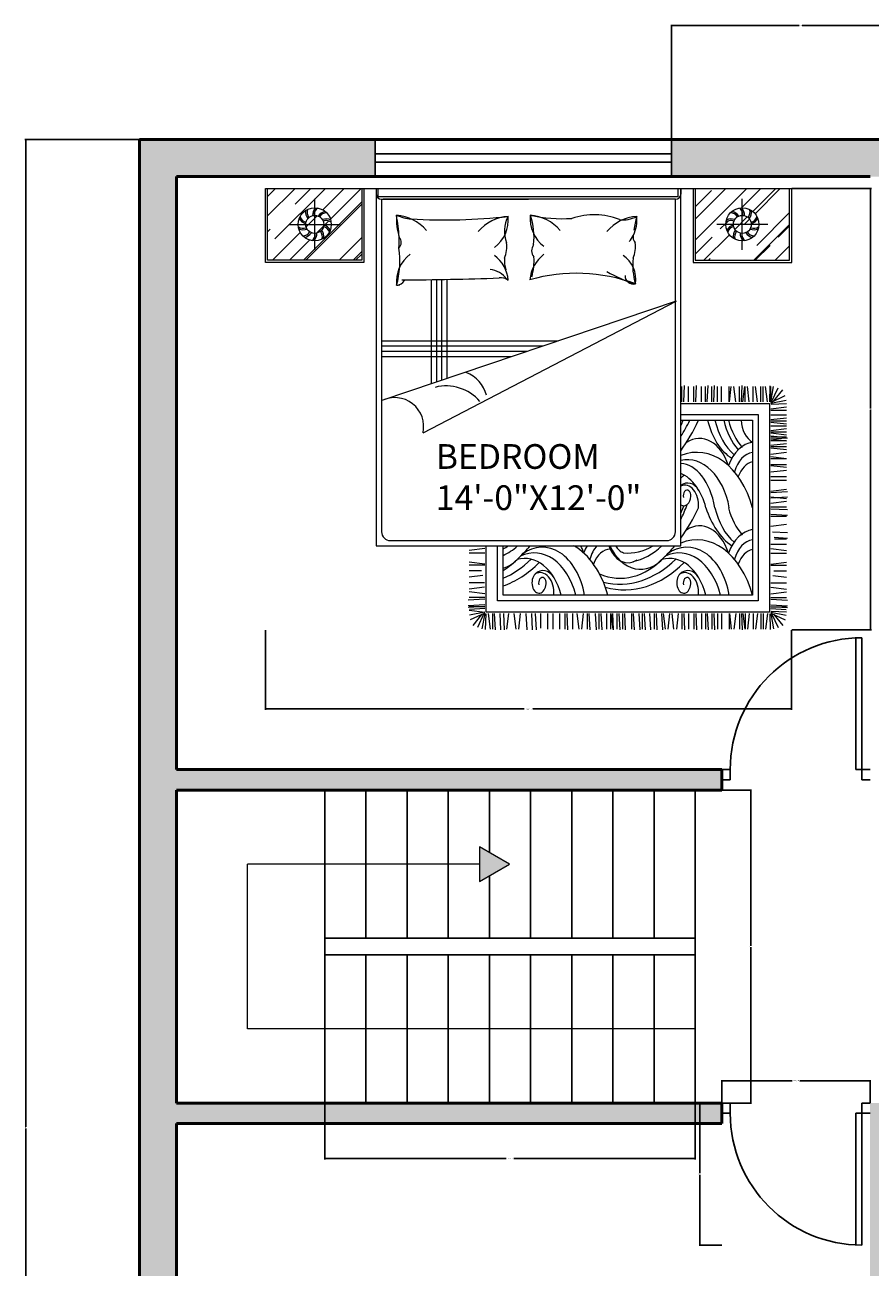
# Model space of a CAD drawing. Units: inches. Extents: x 2831 to 3729, y 3926 to 4974.
# Tile 6 of 8: x 3313 to 3519, y 4672 to 4974. Entities that reach past the tile are written whole.
import ezdxf

# ---------------------------------------------------------------- set-up
doc = ezdxf.new("R2010")
doc.units = ezdxf.units.IN
for name, color, linetype, lineweight in [('A-ANNO-DIMS', 2, 'Continuous', 18), ('A-ANNO-SYMB', 7, 'Continuous', 18), ('A-AREA-IDEN', 7, 'Continuous', 18), ('A-DOOR', 3, 'Continuous', 25), ('A-FLOR-STRS', 7, 'Continuous', 25), ('A-FURN', 8, 'Continuous', 18), ('A-GLAZ', 4, 'Continuous', 25), ('A-WALL', 7, 'Continuous', 50), ('A-WALL-PATT', 252, 'Continuous', 13)]:
    doc.layers.add(name, color=color, linetype=linetype, lineweight=lineweight)
doc.styles.get("Standard").update_dxf_attribs({"font": 'arial.ttf'})
doc.dimstyles.get("Standard").update_dxf_attribs({"dimtxt": 0.18, "dimasz": 0.18, "dimexe": 0.18, "dimexo": 0.0625, "dimgap": 0.09, "dimtad": 0, "dimtih": 1, "dimtoh": 1, "dimdec": 4, "dimzin": 0, "dimdsep": 46, "dimtxsty": 'Standard', "dimcen": 0.09, "dimadec": 0, "dimazin": 0, "dimtfac": 1, "dimtdec": 4, "dimtofl": 0, "dimtmove": 0, "dimatfit": 3, "dimfxl": 1, "dimtolj": 1, "dimtzin": 0, "dimarcsym": 0})

# ---------------------------------------------------------------- blocks, each defined once
blk = doc.blocks.new('A$C64B41DC1')
for p, q in [((0, 2.5079), (2.9903, 2.5079)), ((0, 2.0879), (0, 2.5079)), ((0.012, 2.4618), (0.0581, 2.5079)), ((0.012, 2.3515), (0.1684, 2.5079)), ((0.012, 2.0999), (0.012, 2.5079)), ((0.0543, 2.2213), (0.3409, 2.5079)), ((0.1689, 2.4179), (0.2589, 2.5079)), ((0.3265, 2.386), (0.4484, 2.5079)), ((0.3699, 2.3332), (0.5445, 2.5079)), ((0.548, 2.5079), (0.548, 2.0999)), ((0.56, 2.5079), (0.56, 2.0879)), ((0.6301, 2.5079), (0.6301, 0.4779)), ((0.6401, 2.461), (0.6401, 2.5079)), ((0.6401, 2.5079), (2.344, 2.5079)), ((2.344, 2.5079), (2.3601, 2.5079)), ((2.344, 2.5079), (2.344, 2.461)), ((2.3601, 2.5079), (2.3601, 2.4761)), ((2.3601, 0.4779), (2.3601, 2.5079)), ((2.4303, 2.5079), (2.4303, 2.0879)), ((2.4423, 2.5079), (2.4423, 2.0999)), ((2.4423, 2.3333), (2.6169, 2.5079)), ((2.4423, 2.2145), (2.7357, 2.5079)), ((2.4423, 2.404), (2.5354, 2.4971)), ((2.705, 2.398), (2.8149, 2.5079)), ((2.7691, 2.3772), (2.8998, 2.5079)), ((2.7819, 2.3646), (2.9252, 2.5079)), ((2.9783, 2.0999), (2.9783, 2.5079)), ((2.9903, 2.0879), (2.9903, 2.5079)), ((0.2157, 2.0999), (0.548, 2.4322)), ((0.2299, 2.0999), (0.548, 2.418)), ((0.2804, 2.1597), (0.2804, 2.4481)), ((2.344, 2.461), (0.6401, 2.461)), ((0.6601, 2.4461), (1.4951, 2.4461)), ((0.6601, 2.4461), (0.6601, 0.5579)), ((1.4951, 2.4461), (0.6697, 2.4461)), ((2.3301, 2.4461), (1.4951, 2.4461)), ((2.3301, 0.5579), (2.3301, 2.4461)), ((2.7099, 2.1597), (2.7099, 2.4481)), ((0.2311, 2.2906), (0.2937, 2.3532)), ((2.6674, 2.2756), (2.7382, 2.3464)), ((2.7249, 2.3076), (2.7512, 2.3339)), ((2.7914, 2.1846), (2.9783, 2.3715)), ((0.012, 2.261), (0.0275, 2.2765)), ((0.1362, 2.3039), (0.4246, 2.3039)), ((0.2905, 2.2539), (0.3304, 2.2938)), ((0.3405, 2.3039), (0.3605, 2.3238)), ((2.8541, 2.3039), (2.5657, 2.3039)), ((2.5849, 2.2779), (2.6158, 2.3088)), ((2.6158, 2.3088), (2.6313, 2.3243)), ((2.7746, 2.0999), (2.9783, 2.3036)), ((2.9144, 2.2312), (2.9783, 2.2951)), ((0.0404, 2.0999), (0.1982, 2.2578)), ((0.1365, 2.0999), (0.251, 2.2144)), ((0.4194, 2.0999), (0.548, 2.2285)), ((2.4423, 2.1353), (2.5382, 2.2312)), ((2.4918, 2.0999), (2.6366, 2.2447)), ((0.4986, 2.0999), (0.548, 2.1493)), ((0.5127, 2.0999), (0.548, 2.1352)), ((2.7831, 2.0999), (2.8678, 2.1846)), ((2.8962, 2.0999), (2.9783, 2.182)), ((0.56, 2.0879), (0, 2.0879)), ((0.548, 2.0999), (0.012, 2.0999)), ((2.4303, 2.0879), (2.9903, 2.0879)), ((2.4423, 2.0999), (2.9783, 2.0999)), ((2.5172, 2.0999), (2.5269, 2.1096)), ((0.9415, 1.9902), (0.9415, 1.3975)), ((0.9715, 1.9906), (0.9715, 1.4076)), ((1.0015, 1.991), (1.0015, 1.4177)), ((1.0315, 1.9916), (1.0315, 1.4279)), ((2.3349, 1.8678), (0.6613, 1.3029)), ((0.8956, 1.1191), (2.3349, 1.8678)), ((1.6636, 1.6412), (0.6601, 1.6412)), ((1.5748, 1.6112), (0.6601, 1.6112)), ((2.3665, 1.295), (2.3665, 1.3839)), ((2.377, 1.295), (2.3822, 1.3891)), ((2.4032, 1.295), (2.4032, 1.3839)), ((2.4346, 1.295), (2.4346, 1.3839)), ((2.4451, 1.295), (2.4503, 1.3891)), ((2.4774, 1.2957), (2.4774, 1.3837)), ((2.5, 1.295), (2.5, 1.3839)), ((2.5105, 1.295), (2.5157, 1.3891)), ((2.5367, 1.295), (2.5367, 1.3839)), ((2.5471, 1.295), (2.5524, 1.3891)), ((2.5681, 1.295), (2.5681, 1.3839)), ((2.5918, 1.295), (2.5918, 1.3839)), ((2.6346, 1.2957), (2.6346, 1.3837)), ((2.6362, 1.2957), (2.6467, 1.3839)), ((2.6729, 1.295), (2.6624, 1.3839)), ((2.6938, 1.295), (2.6938, 1.3839)), ((2.7043, 1.295), (2.7095, 1.3891)), ((2.7127, 1.2957), (2.7232, 1.3839)), ((2.7253, 1.295), (2.7253, 1.3839)), ((2.7494, 1.295), (2.7389, 1.3839)), ((2.7718, 1.295), (2.7718, 1.3839)), ((2.7959, 1.295), (2.7854, 1.3839)), ((2.8146, 1.2957), (2.8146, 1.3837)), ((2.8146, 1.2957), (2.8146, 1.3837)), ((2.8282, 1.295), (2.8282, 1.3839)), ((2.8282, 1.295), (2.8282, 1.3839)), ((2.8523, 1.295), (2.8418, 1.3839)), ((2.8523, 1.295), (2.8418, 1.3839)), ((2.8653, 1.2966), (2.8688, 1.3861)), ((2.8711, 1.2957), (2.8711, 1.3837)), ((2.8711, 1.2957), (2.8875, 1.3822)), ((2.8765, 1.2958), (2.9132, 1.3758)), ((2.8893, 1.3011), (2.9394, 1.3636)), ((2.3601, 1.2873), (2.8639, 1.2873)), ((2.8639, 1.2873), (2.8639, 0.1018)), ((2.8713, 1.2927), (2.954, 1.3315)), ((2.8717, 1.2884), (2.9588, 1.3058)), ((2.8744, 1.2817), (2.9603, 1.2869)), ((2.3601, 1.2233), (2.7999, 1.2233)), ((2.7999, 1.2233), (2.7999, 0.1658)), ((2.8716, 1.2565), (2.9605, 1.2669)), ((2.8716, 1.2212), (2.9605, 1.2212)), ((2.8716, 1.1947), (2.9605, 1.2052)), ((2.8723, 1.2489), (2.9603, 1.2489)), ((2.3601, 1.1913), (2.7679, 1.1912)), ((2.7679, 1.1912), (2.7679, 0.1978)), ((2.8716, 1.181), (2.9605, 1.1705)), ((2.8716, 1.1595), (2.9605, 1.1595)), ((2.8716, 1.133), (2.9605, 1.1435)), ((2.8723, 1.1872), (2.9603, 1.1872)), ((2.8716, 1.1193), (2.9605, 1.1088)), ((2.8716, 1.1035), (2.9605, 1.093)), ((2.8716, 1.0965), (2.9605, 1.0965)), ((2.8716, 1.086), (2.9657, 1.0913)), ((2.8716, 1.0756), (2.9605, 1.0756)), ((2.8716, 1.0491), (2.9605, 1.0596)), ((2.8723, 1.1255), (2.9603, 1.1255)), ((2.8723, 1.0858), (2.9605, 1.0753)), ((2.8716, 1.0354), (2.9605, 1.0249)), ((2.8723, 1.0416), (2.9603, 1.0416)), ((2.8723, 0.9987), (2.9605, 1.0092)), ((2.8716, 0.9346), (2.9605, 0.9241)), ((2.8723, 0.985), (2.9605, 0.9745)), ((2.8723, 0.9735), (2.9603, 0.9735)), ((2.8723, 0.9408), (2.9603, 0.9408)), ((2.8723, 0.8979), (2.9605, 0.9084)), ((2.8723, 0.8726), (2.9603, 0.8726)), ((2.8723, 0.8505), (2.9603, 0.8505)), ((2.8716, 0.7885), (2.9605, 0.799)), ((2.8716, 0.7818), (2.9657, 0.787)), ((2.8716, 0.7503), (2.9657, 0.7556)), ((2.8716, 0.7204), (2.9605, 0.7309)), ((2.8723, 0.7571), (2.9605, 0.7466)), ((2.8716, 0.6995), (2.9605, 0.6995)), ((2.8716, 0.689), (2.9657, 0.6838)), ((2.8716, 0.6576), (2.9657, 0.6523)), ((2.8716, 0.6471), (2.9605, 0.6471)), ((2.8716, 0.5903), (2.9605, 0.6007)), ((0.7101, 0.5079), (2.2801, 0.5079)), ((2.882, 0.5582), (2.9657, 0.5536)), ((2.8909, 0.5263), (2.9657, 0.5222)), ((2.8928, 0.5169), (2.9605, 0.5169)), ((0.6301, 0.4779), (2.3601, 0.4779)), ((1.2465, 0.4625), (1.1576, 0.452)), ((1.2465, 0.4365), (1.1577, 0.4365)), ((1.2542, 0.1018), (1.2542, 0.4779)), ((1.3182, 0.1658), (1.3182, 0.4779)), ((1.3502, 0.1978), (1.3502, 0.4779)), ((2.8716, 0.4877), (2.9603, 0.4877)), ((2.8716, 0.4625), (2.9605, 0.452)), ((2.8716, 0.4365), (2.9603, 0.4365)), ((1.2465, 0.3746), (1.1576, 0.3851)), ((1.2465, 0.3684), (1.1577, 0.3684)), ((2.8716, 0.3746), (2.9605, 0.3851)), ((2.8716, 0.3684), (2.9603, 0.3684)), ((1.2355, 0.3092), (1.1576, 0.3)), ((1.2285, 0.3357), (1.1577, 0.3357)), ((2.8826, 0.3092), (2.9605, 0.3)), ((2.8896, 0.3357), (2.9603, 0.3357)), ((1.2457, 0.2423), (1.1576, 0.2319)), ((1.2465, 0.2057), (1.1576, 0.2161)), ((1.2457, 0.2676), (1.1577, 0.2676)), ((2.8716, 0.2057), (2.9605, 0.2161)), ((2.8723, 0.2676), (2.9603, 0.2676)), ((2.8723, 0.2423), (2.9605, 0.2319)), ((1.2465, 0.1742), (1.1524, 0.169)), ((1.2465, 0.1428), (1.1524, 0.1376)), ((1.2465, 0.1847), (1.1576, 0.1847)), ((2.7999, 0.1658), (1.3182, 0.1658)), ((2.7679, 0.1978), (1.3502, 0.1978)), ((2.8716, 0.1847), (2.9605, 0.1847)), ((2.8716, 0.1742), (2.9657, 0.169)), ((2.8716, 0.1428), (2.9657, 0.1376)), ((1.2465, 0.1334), (1.1524, 0.1281)), ((1.2465, 0.1323), (1.1576, 0.1323)), ((1.2465, 0.1323), (1.1576, 0.1323)), ((1.2465, 0.1), (1.1576, 0.1105)), ((1.2465, 0.1229), (1.1588, 0.1168)), ((1.2464, 0.1007), (1.1592, 0.0833)), ((1.2468, 0.0964), (1.1641, 0.0576)), ((1.2288, 0.088), (1.1787, 0.0255)), ((1.2415, 0.0933), (1.2049, 0.0133)), ((1.247, 0.0934), (1.2306, 0.0069)), ((1.2527, 0.0925), (1.2493, 0.003)), ((2.8639, 0.1018), (1.2542, 0.1018)), ((1.2658, 0.0941), (1.2762, 0.0052)), ((1.2899, 0.0941), (1.2899, 0.0052)), ((1.2999, 0.0941), (1.3051, 0)), ((1.3313, 0.0941), (1.3365, 0)), ((1.3523, 0.0941), (1.3575, 0)), ((1.3804, 0.0941), (1.3699, 0.0052)), ((1.4119, 0.0934), (1.4223, 0.0052)), ((1.4485, 0.0941), (1.438, 0.0052)), ((1.48, 0.0941), (1.4852, 0)), ((1.5114, 0.0941), (1.5166, 0)), ((1.5323, 0.0941), (1.5376, 0)), ((1.5638, 0.0941), (1.5638, 0.0105)), ((1.6021, 0.0941), (1.6021, 0.0052)), ((1.6336, 0.0941), (1.6336, 0.0052)), ((1.6702, 0.0941), (1.6702, 0.0052)), ((1.7017, 0.0941), (1.7017, 0.0052)), ((1.7122, 0.0941), (1.7174, 0)), ((1.7445, 0.0934), (1.7445, 0.0054)), ((1.7698, 0.0934), (1.7803, 0.0052)), ((1.8065, 0.0941), (1.796, 0.0052)), ((1.8274, 0.0941), (1.8274, 0.0052)), ((1.8379, 0.0941), (1.8431, 0)), ((1.8746, 0.0941), (1.8798, 0)), ((1.8955, 0.0941), (1.8955, 0.0052)), ((1.906, 0.0941), (1.9113, 0)), ((1.9384, 0.0934), (1.9384, 0.0054)), ((1.9609, 0.0941), (1.9609, 0.0052)), ((1.9636, 0.0934), (1.9741, 0.0052)), ((1.9714, 0.0941), (1.9766, 0)), ((1.9976, 0.0941), (1.9976, 0.0052)), ((2.0081, 0.0941), (2.0133, 0)), ((2.029, 0.0941), (2.029, 0.0052)), ((2.0395, 0.0941), (2.0447, 0)), ((2.0797, 0.0941), (2.0797, 0.0052)), ((2.0902, 0.0941), (2.0954, 0)), ((2.1216, 0.0941), (2.1269, 0)), ((2.1412, 0.0941), (2.1412, 0.0052)), ((2.1517, 0.0941), (2.1569, 0)), ((2.1831, 0.0941), (2.1884, 0)), ((2.2093, 0.0941), (2.2093, 0.0052)), ((2.2198, 0.0941), (2.225, 0)), ((2.2512, 0.0941), (2.2565, 0)), ((2.2603, 0.0934), (2.2707, 0.0052)), ((2.2969, 0.0941), (2.2864, 0.0052)), ((2.3089, 0.0934), (2.3193, 0.0052)), ((2.3455, 0.0941), (2.3351, 0.0052)), ((2.3665, 0.0941), (2.3665, 0.0052)), ((2.377, 0.0941), (2.3822, 0)), ((2.4032, 0.0941), (2.4032, 0.0052)), ((2.4346, 0.0941), (2.4346, 0.0052)), ((2.4451, 0.0941), (2.4503, 0)), ((2.4774, 0.0934), (2.4774, 0.0054)), ((2.5, 0.0941), (2.5, 0.0052)), ((2.5105, 0.0941), (2.5157, 0)), ((2.5367, 0.0941), (2.5367, 0.0052)), ((2.5471, 0.0941), (2.5524, 0)), ((2.5681, 0.0941), (2.5681, 0.0052)), ((2.5918, 0.0941), (2.5918, 0.0052)), ((2.6346, 0.0934), (2.6346, 0.0054)), ((2.6362, 0.0934), (2.6467, 0.0052)), ((2.6729, 0.0941), (2.6624, 0.0052)), ((2.6938, 0.0941), (2.6938, 0.0052)), ((2.7043, 0.0941), (2.7095, 0)), ((2.7127, 0.0934), (2.7232, 0.0052)), ((2.7253, 0.0941), (2.7253, 0.0052)), ((2.7494, 0.0941), (2.7389, 0.0052)), ((2.7718, 0.0941), (2.7718, 0.0052)), ((2.7959, 0.0941), (2.7854, 0.0052)), ((2.8146, 0.0934), (2.8146, 0.0054)), ((2.8282, 0.0941), (2.8282, 0.0052)), ((2.8523, 0.0941), (2.8418, 0.0052)), ((2.8653, 0.0925), (2.8688, 0.003)), ((2.8711, 0.0934), (2.8875, 0.0069)), ((2.8713, 0.0964), (2.954, 0.0576)), ((2.8716, 0.1334), (2.9657, 0.1281)), ((2.8716, 0.1323), (2.9605, 0.1323)), ((2.8716, 0.1229), (2.9593, 0.1168)), ((2.8717, 0.1007), (2.9588, 0.0833)), ((2.8744, 0.1074), (2.9603, 0.1022)), ((2.8765, 0.0933), (2.9132, 0.0133)), ((2.8893, 0.088), (2.9394, 0.0255))]:
    blk.add_line(p, q)
at = {"ltscale": 10}
for p, q in [((1.4859, 1.5812), (0.6601, 1.5812)), ((1.397, 1.5512), (0.6601, 1.5512))]:
    blk.add_line(p, q, dxfattribs=at)
for centre, radius in [((0.2804, 2.3039), 0.0942), ((0.2804, 2.3039), 0.051), ((2.7099, 2.3039), 0.0942), ((2.7099, 2.3039), 0.051)]:
    blk.add_circle(centre, radius)
for centre, radius, start, end in [((0.6601, 2.4761), 0.03, 180, 270), ((2.3301, 2.4761), 0.03, 270, 0), ((0.2457, 2.3659), 0.0605, 208.17003, 254.48975), ((0.2417, 2.3614), 0.0462, 196.30017, 256.53802), ((0.2887, 2.3745), 0.0605, 172.17003, 218.48975), ((0.2828, 2.3731), 0.0462, 160.30017, 220.53802), ((0.3286, 2.3561), 0.0605, 136.17003, 182.48975), ((0.3231, 2.3585), 0.0462, 124.30017, 184.53802), ((0.3501, 2.3178), 0.0605, 100.17003, 146.48975), ((0.347, 2.323), 0.0462, 88.30017, 148.53802), ((0.3449, 2.2742), 0.0605, 64.17003, 110.48975), ((1.0526, 2.3302), 0.3085, 175.30484, 198.69419), ((-0.8702, 2.0941), 1.6364, 4.80985, 9.18918), ((0.8579, 2.6278), 0.2948, 247.51785, 264.26696), ((0.728, 2.111), 0.245, 40.4189, 85.9871), ((1.0164, 5.7096), 3.3803, 266.81337, 276.16021), ((1.3963, 2.1044), 0.245, 94.0129, 139.5811), ((1.1858, 2.3288), 0.1943, 306.5711, 5.88998), ((1.5348, 2.2652), 0.1767, 151.77364, 201.69827), ((1.6986, 2.3355), 0.1943, 174.11002, 233.4289), ((1.1481, 2.2311), 0.3783, 353.49469, 19.18669), ((1.6871, 3.192), 0.8561, 257.74383, 273.62843), ((1.4882, 2.111), 0.245, 40.4189, 85.9871), ((1.8674, 1.9709), 0.3878, 68.20259, 108.9817), ((2.1269, 2.1044), 0.245, 94.0129, 139.5811), ((2.0342, 2.4856), 0.1563, 261.59582, 298.90918), ((1.9165, 2.3288), 0.1943, 333.73715, 5.88998), ((2.6058, 2.2028), 0.517, 163.60457, 172.3273), ((2.6454, 2.2742), 0.0605, 69.51025, 115.82997), ((2.6433, 2.323), 0.0462, 31.46198, 91.69983), ((2.6402, 2.3178), 0.0605, 33.51025, 79.82997), ((2.6672, 2.3585), 0.0462, 355.46198, 55.69983), ((2.6617, 2.3561), 0.0605, 357.51025, 43.82997), ((2.7075, 2.3731), 0.0462, 319.46198, 19.69983), ((2.7016, 2.3745), 0.0605, 321.51025, 7.82997), ((2.7486, 2.3614), 0.0462, 283.46198, 343.69983), ((2.7446, 2.3659), 0.0605, 285.51025, 331.82997), ((0.2153, 2.3276), 0.0462, 232.30017, 292.53802), ((0.2158, 2.3336), 0.0605, 244.17003, 290.48975), ((0.2138, 2.2848), 0.0462, 268.30017, 328.53802), ((0.2779, 2.2347), 0.0462, 340.30017, 40.53802), ((0.272, 2.2333), 0.0605, 352.17003, 38.48975), ((0.3455, 2.2802), 0.0462, 52.30017, 112.53802), ((0.3191, 2.2464), 0.0462, 16.30017, 76.53802), ((0.3151, 2.2419), 0.0605, 28.17003, 74.48975), ((2.6448, 2.2802), 0.0462, 67.46198, 127.69983), ((2.6752, 2.2419), 0.0605, 105.51025, 151.82997), ((2.6712, 2.2464), 0.0462, 103.46198, 163.69983), ((2.7182, 2.2333), 0.0605, 141.51025, 187.82997), ((2.7123, 2.2347), 0.0462, 139.46198, 199.69983), ((2.7765, 2.2848), 0.0462, 211.46198, 271.69983), ((2.7744, 2.3336), 0.0605, 249.51025, 295.82997), ((2.775, 2.3276), 0.0462, 247.46198, 307.69983), ((0.2107, 2.29), 0.0605, 280.17003, 326.48975), ((0.2377, 2.2493), 0.0462, 304.30017, 4.53802), ((0.2322, 2.2517), 0.0605, 316.17003, 2.48975), ((0.7274, 2.2013), 0.0446, 314.4736, 42.17134), ((-1.6008, 2.277), 2.3618, 357.39054, 358.88764), ((1.204, 2.1778), 0.1681, 337.01697, 7.53676), ((1.5671, 2.1546), 0.0547, 142.08329, 220.902), ((1.9165, 2.3288), 0.1943, 320.94042, 333.73715), ((2.1347, 2.2313), 0.0459, 165.35061, 223.26844), ((1.9346, 2.1778), 0.1681, 337.01697, 7.53676), ((2.7581, 2.2517), 0.0605, 177.51025, 223.82997), ((2.7526, 2.2493), 0.0462, 175.46198, 235.69983), ((2.7796, 2.29), 0.0605, 213.51025, 259.82997), ((0.9385, 1.978), 0.1943, 126.5711, 185.88998), ((0.2688, 2.0945), 0.4956, 344.0243, 8.70709), ((1.1858, 1.9714), 0.1943, 4.31813, 53.4289), ((1.7059, 1.9714), 0.204, 127.11975, 175.09005), ((1.1965, 2.0983), 0.3299, 343.79543, 3.55541), ((1.9394, 1.991), 0.1651, 351.26213, 55.75721), ((1.2687, 1.9248), 0.1223, 33.62799, 86.47438), ((1.5415, 2.0969), 0.1834, 175.22328, 196.23004), ((2.4617, 2.0719), 0.3745, 173.82958, 196.4356), ((0.7417, 2.0149), 0.057, 273.47085, 328.54118), ((0.7246, 18.8439), 16.8552, 270.17399, 272.05214), ((1.3401, 1.9404), 0.0603, 49.09906, 101.37023), ((1.7676, 1.0629), 0.9631, 69.65065, 105.96307), ((2.2748, 2.5795), 0.6373, 238.34989, 254.31375), ((2.0911, 2.0123), 0.0478, 179.77267, 283.80184), ((0.728, 2.2025), 0.245, 274.0129, 278.34166), ((1.0747, 1.2871), 0.1871, 14.1863, 69.12121), ((1.0274, 1.1334), 0.2527, 40.62904, 104.37123), ((0.7347, 1.1553), 0.1649, 347.31088, 116.44537), ((0.7101, 0.5579), 0.05, 180, 270), ((2.2801, 0.5579), 0.05, 270, 0)]:
    blk.add_arc(centre, radius, start, end)
for centre, major_axis, ratio, start_param, end_param in [((1.9938, 1.6262), (0, -0.7531), 0.68, 0.797284, 0.954936), ((2.0643, 1.466), (0, -0.5322), 0.68, 7.239912, 7.311536), ((1.9052, 1.7397), (0, -0.9842), 0.68, 0.74745, 0.979724), ((2.7455, 1.3081), (0, 0.3614), 0.68, 1.900046, 2.742661), ((2.7868, 1.3081), (0, 0.3614), 0.68, 1.900046, 2.614747), ((2.8372, 1.3081), (0, 0.3614), 0.68, 1.900046, 2.479658), ((2.8607, 1.3211), (0, 0.3614), 0.68, 1.938265, 2.479658), ((2.8057, 1.2079), (0, -0.1524), 0.68, 4.821745, 5.895886), ((2.4513, 0.5069), (0, 0.502), 0.68, 5.095327, 6.553458), ((2.4665, 0.8216), (0, -0.2664), 0.68, 2.006169, 3.565187), ((2.7862, 0.8069), (0, -0.2615), 0.68, 3.244645, 4.205018), ((2.396, 0.6032), (0, 0.3641), 0.68, -1.3172, 0.145284), ((2.7784, 0.8289), (0, -0.1802), 0.68, 3.227058, 4.318474), ((2.3507, 0.5642), (0.0073, 0.3819), 0.56205, -1.21172, -0.009991), ((2.7821, 0.7971), (0, -0.1589), 0.68, 3.272942, 4.229533), ((2.2964, 0.5771), (0, -0.3263), 0.68, 1.938944, 2.850232), ((2.0403, 1.6015), (0, -0.8763), 0.68, 6.849801, 6.887077), ((2.4005, 0.7132), (0, -0.1214), 0.68, 2.284368, 3.652258), ((2.3834, 0.7081), (0, 0.1147), 0.68, 4.593909, 6.585576), ((2.3961, 0.7628), (0, -0.0317), 0.68, 1.462497, 5.046281), ((2.3774, 0.7653), (0, -0.0593), 0.68, 5.841311, 7.755362), ((1.9938, 1.1295), (-0.0678, 0.7439), 0.610498, 3.917146, 4.063997), ((2.0643, 0.9693), (0, -0.5322), 0.68, 7.239912, 7.336618), ((1.9052, 1.243), (0, -0.9842), 0.68, 0.74745, 0.979724), ((2.7455, 0.8114), (-0.0599, 0.3735), 0.695517, 1.775813, 2.548612), ((2.7868, 0.8114), (0, 0.3614), 0.68, 1.900046, 2.614747), ((2.8607, 0.8243), (0, 0.3614), 0.68, 1.938265, 2.479658), ((2.4665, 0.3249), (0, -0.2664), 0.68, 2.006169, 3.565187), ((2.7862, 0.3102), (0, -0.2615), 0.68, 3.244645, 4.205018), ((2.4513, 0.0102), (0, 0.502), 0.68, 5.095327, 6.553458), ((2.7784, 0.3322), (0, -0.1802), 0.68, 3.227058, 4.318474), ((1.242, 0.9693), (0, -0.5322), 0.68, 6.586764, 6.677612), ((1.1714, 1.1295), (-0.1157, 0.7241), 0.59432, 3.291697, 3.50733), ((1.474, 0.0804), (0, -0.3263), 0.68, 1.938944, 3.339184), ((1.0828, 1.243), (0, -0.9842), 0.68, 0.565948, 0.680366), ((1.5283, 0.0674), (0, -0.3703), 0.68, 1.930561, 3.464283), ((1.5736, 0.1065), (0, 0.3641), 0.68, -1.3172, 0.476403), ((1.6289, 0.0102), (0, 0.502), 0.68, 6.655152, 6.661293), ((1.6289, 0.0102), (0, 0.502), 0.68, 5.095327, 5.911219), ((1.6442, 0.3249), (0, -0.2664), 0.68, 2.006169, 2.182797), ((1.9638, 0.3102), (0, -0.2615), 0.68, 4.015924, 4.205018), ((1.956, 0.3322), (0, -0.1802), 0.68, 3.770744, 4.318474), ((1.9597, 0.3004), (0, -0.1589), 0.68, 3.14258, 4.229533), ((2.0606, 0.5616), (0, -0.1803), 0.68, 5.194792, 5.929328), ((2.0606, 0.5616), (0, -0.1803), 0.68, 5.194792, 6.723255), ((2.1315, 0.6603), (0, -0.3155), 0.68, 5.328638, 6.949396), ((2.0549, 0.5656), (0, -0.1303), 0.68, 5.450951, 6.054641), ((2.0643, 0.9693), (0, -0.5322), 0.68, 6.20013, 6.677612), ((1.9938, 1.1295), (-0.0678, 0.7439), 0.610498, 3.199135, 3.592282), ((2.2964, 0.0804), (0, -0.3263), 0.68, 1.938944, 3.339184), ((1.9052, 1.243), (0, -0.9842), 0.68, 0.565948, 0.680366), ((2.3507, 0.0674), (0, -0.3703), 0.68, 1.930561, 3.464283), ((2.396, 0.1065), (0, 0.3641), 0.68, -1.3172, 0.476403), ((2.4513, 0.0102), (0, 0.502), 0.68, 6.655152, 6.661293), ((2.7821, 0.3004), (0, -0.1589), 0.68, 3.272942, 4.229533), ((1.1933, 0.9181), (0, -0.624), 0.68, 0.378672, 0.625379), ((1.3091, 0.6603), (0, -0.3155), 0.68, 6.475719, 6.949396), ((1.1911, 1.1066), (0, 0.8458), 0.68, 3.421828, 3.728616), ((1.2179, 1.1047), (0, -0.8763), 0.68, 6.507006, 6.887077), ((2.0157, 0.9181), (0, -0.624), 0.68, -0.280078, 0.625379), ((2.0135, 1.1066), (0, 0.8458), 0.68, 2.978727, 3.728616), ((2.0403, 1.1047), (0, -0.8763), 0.68, 6.099302, 6.887077), ((1.555, 0.2685), (0, -0.0593), 0.68, 3.732151, 7.755362), ((1.5781, 0.2165), (0, -0.1214), 0.68, 2.284368, 3.726131), ((1.561, 0.2114), (0, 0.1147), 0.68, 4.593909, 6.647252), ((1.5737, 0.2661), (0, -0.0317), 0.68, 1.462497, 5.046281), ((2.3774, 0.2685), (0, -0.0593), 0.68, 3.732151, 7.755362), ((2.4005, 0.2165), (0, -0.1214), 0.68, 2.284368, 3.726131), ((2.3834, 0.2114), (0, 0.1147), 0.68, 4.593909, 6.647252), ((2.3961, 0.2661), (0, -0.0317), 0.68, 1.462497, 5.046281)]:
    blk.add_ellipse(centre, major_axis=major_axis, ratio=ratio, start_param=start_param, end_param=end_param)
blk = doc.blocks.new('DOOR-SWING-32IN')
for p, q in [((-32, 2.5), (-34, 2.5)), ((-34, 0), (-32, 0)), ((-32, 0), (-32, 2.5)), ((0, 0), (0, 2.5)), ((0, 2.5), (2, 2.5)), ((2, 0), (0, 0)), ((-1.5, 0), (-1.5, -31.96)), ((0, 0), (-1.5, 0)), ((0, 0), (0, -32))]:
    blk.add_line(p, q)
blk.add_arc((0, 0), 32, 180, 270)
blk = doc.blocks.new('WINDOW-72IN-PLAN')
for p, q in [((0, 0), (0, 9)), ((72, 0), (72, 9)), ((72, 5.5), (0, 5.5)), ((72, 3.5), (0, 3.5))]:
    blk.add_line(p, q)
blk = doc.blocks.new('STAIR-HALF-TURN')
for p, q in [((0, 76), (0, 40)), ((10, 76), (10, 40)), ((20, 76), (20, 40)), ((30, 76), (30, 40)), ((40, 76), (40, 60.82)), ((50, 76), (50, 40)), ((60, 76), (60, 40)), ((70, 76), (70, 40)), ((80, 76), (80, 40)), ((90, 76), (90, 40)), ((40, 55.18), (40, 40)), ((90, 40), (0, 40)), ((0, 36), (0, 40)), ((90, 36), (90, 40)), ((90, 36), (0, 36)), ((0, 36), (0, 0)), ((10, 36), (10, 0)), ((20, 36), (20, 0)), ((30, 36), (30, 0)), ((40, 36), (40, 0)), ((50, 36), (50, 0)), ((60, 36), (60, 0)), ((70, 36), (70, 0)), ((80, 36), (80, 0)), ((90, 36), (90, 0))]:
    blk.add_line(p, q)
blk = doc.blocks.new('STAIR-DIRECTION')
h = blk.add_hatch(color=256)
h.dxf.hatch_style = 1
h.paths.add_polyline_path([(63.65, 40), (56.32, 44.24), (56.32, 35.76)])
for p, q in [((0, 0), (0, 40)), ((56.32, 40), (0, 40)), ((108.76, 0), (0, 0))]:
    blk.add_line(p, q)
blk.add_lwpolyline([(63.65, 40), (56.32, 44.24), (56.32, 35.76)], close=True)
blk = doc.blocks.new('*D17')
at = {"layer": 'A-ANNO-DIMS', "color": 0, "lineweight": -2, "transparency": 16777216}
for p, q in [((3482.81, 4712.2), (3482.81, 4717.72)), ((3482.99, 4717.54), (3499.87, 4717.54)), ((3518.63, 4717.54), (3501.74, 4717.54)), ((3518.81, 4712.2), (3518.81, 4717.72))]:
    blk.add_line(p, q, dxfattribs=at)
at = {"layer": 'A-ANNO-DIMS', "color": 0, "transparency": 16777216}
for points in [[(3482.99, 4717.57), (3482.99, 4717.51), (3482.81, 4717.54)], [(3518.63, 4717.57), (3518.63, 4717.51), (3518.81, 4717.54)]]:
    blk.add_solid(points, dxfattribs=at)
at = {"layer": 'Defpoints', "color": 0, "transparency": 16777216}
for p in [(3518.81, 4717.54), (3482.81, 4712.14), (3518.81, 4712.14)]:
    blk.add_point(p, dxfattribs=at)
at = {"layer": 'A-ANNO-DIMS', "color": 0, "transparency": 16777216, "insert": (3500.81, 4717.54), "char_height": 0.18, "attachment_point": 5}
blk.add_mtext('\\A1;DOOR 36 TYP.', dxfattribs=at)
blk = doc.blocks.new('*D18')
at = {"layer": 'A-ANNO-DIMS', "color": 0, "lineweight": -2, "transparency": 16777216}
for p, q in [((3482.75, 4712.14), (3477.23, 4712.14)), ((3477.41, 4711.96), (3477.41, 4695.07)), ((3477.41, 4677.82), (3477.41, 4694.71)), ((3482.75, 4677.64), (3477.23, 4677.64))]:
    blk.add_line(p, q, dxfattribs=at)
at = {"layer": 'A-ANNO-DIMS', "color": 0, "transparency": 16777216}
for points in [[(3477.38, 4711.96), (3477.44, 4711.96), (3477.41, 4712.14)], [(3477.38, 4677.82), (3477.44, 4677.82), (3477.41, 4677.64)]]:
    blk.add_solid(points, dxfattribs=at)
at = {"layer": 'Defpoints', "color": 0, "transparency": 16777216}
for p in [(3477.41, 4712.14), (3482.81, 4712.14), (3482.81, 4677.64)]:
    blk.add_point(p, dxfattribs=at)
at = {"layer": 'A-ANNO-DIMS', "color": 0, "transparency": 16777216, "insert": (3477.41, 4694.89), "char_height": 0.18, "attachment_point": 5}
blk.add_mtext('\\A1;35 TYP.', dxfattribs=at)
blk = doc.blocks.new('*D29')
at = {"layer": 'A-ANNO-DIMS', "color": 0, "lineweight": -2, "transparency": 16777216}
for p, q in [((3386.31, 4712.08), (3386.31, 4698.46)), ((3476.31, 4712.08), (3476.31, 4698.46)), ((3386.49, 4698.64), (3430.38, 4698.64)), ((3476.13, 4698.64), (3432.24, 4698.64))]:
    blk.add_line(p, q, dxfattribs=at)
at = {"layer": 'A-ANNO-DIMS', "color": 0, "transparency": 16777216}
for points in [[(3386.49, 4698.67), (3386.49, 4698.61), (3386.31, 4698.64)], [(3476.13, 4698.67), (3476.13, 4698.61), (3476.31, 4698.64)]]:
    blk.add_solid(points, dxfattribs=at)
at = {"layer": 'Defpoints', "color": 0, "transparency": 16777216}
for p in [(3386.31, 4712.14), (3476.31, 4712.14), (3476.31, 4698.64)]:
    blk.add_point(p, dxfattribs=at)
at = {"layer": 'A-ANNO-DIMS', "color": 0, "transparency": 16777216, "insert": (3431.31, 4698.64), "char_height": 0.18, "attachment_point": 5}
blk.add_mtext('\\A1;STAIR 90 TYP.', dxfattribs=at)
blk = doc.blocks.new('*D30')
at = {"layer": 'A-ANNO-DIMS', "color": 0, "lineweight": -2, "transparency": 16777216}
for p, q in [((3476.37, 4788.14), (3489.99, 4788.14)), ((3489.81, 4787.96), (3489.81, 4750.32)), ((3489.81, 4712.32), (3489.81, 4749.96)), ((3476.37, 4712.14), (3489.99, 4712.14))]:
    blk.add_line(p, q, dxfattribs=at)
at = {"layer": 'A-ANNO-DIMS', "color": 0, "transparency": 16777216}
for points in [[(3489.78, 4787.96), (3489.84, 4787.96), (3489.81, 4788.14)], [(3489.78, 4712.32), (3489.84, 4712.32), (3489.81, 4712.14)]]:
    blk.add_solid(points, dxfattribs=at)
at = {"layer": 'Defpoints', "color": 0, "transparency": 16777216}
for p in [(3476.31, 4788.14), (3489.81, 4788.14), (3476.31, 4712.14)]:
    blk.add_point(p, dxfattribs=at)
at = {"layer": 'A-ANNO-DIMS', "color": 0, "transparency": 16777216, "insert": (3489.81, 4750.14), "char_height": 0.18, "attachment_point": 5}
blk.add_mtext('\\A1;76 TYP.', dxfattribs=at)
blk = doc.blocks.new('*D31')
at = {"layer": 'A-ANNO-DIMS', "color": 0, "lineweight": -2, "transparency": 16777216}
for p, q in [((3371.89, 4826.95), (3371.89, 4807.66)), ((3499.74, 4826.95), (3499.74, 4807.66)), ((3372.07, 4807.84), (3434.74, 4807.84)), ((3499.56, 4807.84), (3436.89, 4807.84))]:
    blk.add_line(p, q, dxfattribs=at)
at = {"layer": 'A-ANNO-DIMS', "color": 0, "transparency": 16777216}
for points in [[(3372.07, 4807.87), (3372.07, 4807.81), (3371.89, 4807.84)], [(3499.56, 4807.87), (3499.56, 4807.81), (3499.74, 4807.84)]]:
    blk.add_solid(points, dxfattribs=at)
at = {"layer": 'Defpoints', "color": 0, "transparency": 16777216}
for p in [(3371.89, 4827.02), (3499.74, 4827.02), (3499.74, 4807.84)]:
    blk.add_point(p, dxfattribs=at)
at = {"layer": 'A-ANNO-DIMS', "color": 0, "transparency": 16777216, "insert": (3435.82, 4807.84), "char_height": 0.18, "attachment_point": 5}
blk.add_mtext('\\A1;BED GROUP 128', dxfattribs=at)
blk = doc.blocks.new('*D32')
at = {"layer": 'A-ANNO-DIMS', "color": 0, "lineweight": -2, "transparency": 16777216}
for p, q in [((3499.8, 4934.24), (3519.1, 4934.24)), ((3518.92, 4934.06), (3518.92, 4880.81)), ((3518.92, 4827.2), (3518.92, 4880.45)), ((3499.8, 4827.02), (3519.1, 4827.02))]:
    blk.add_line(p, q, dxfattribs=at)
at = {"layer": 'A-ANNO-DIMS', "color": 0, "transparency": 16777216}
for points in [[(3518.89, 4934.06), (3518.95, 4934.06), (3518.92, 4934.24)], [(3518.89, 4827.2), (3518.95, 4827.2), (3518.92, 4827.02)]]:
    blk.add_solid(points, dxfattribs=at)
at = {"layer": 'Defpoints', "color": 0, "transparency": 16777216}
for p in [(3499.74, 4934.24), (3518.92, 4934.24), (3499.74, 4827.02)]:
    blk.add_point(p, dxfattribs=at)
at = {"layer": 'A-ANNO-DIMS', "color": 0, "transparency": 16777216, "insert": (3518.92, 4880.63), "char_height": 0.18, "attachment_point": 5}
blk.add_mtext('\\A1;107', dxfattribs=at)
blk = doc.blocks.new('*D55')
at = {"layer": 'A-ANNO-DIMS', "color": 0, "lineweight": -2, "transparency": 16777216}
for p, q in [((3341.25, 4946.14), (3313.48, 4946.14)), ((3313.66, 4945.96), (3313.66, 4706.32)), ((3313.66, 4466.32), (3313.66, 4705.96)), ((3518.75, 4466.14), (3313.48, 4466.14))]:
    blk.add_line(p, q, dxfattribs=at)
at = {"layer": 'A-ANNO-DIMS', "color": 0, "transparency": 16777216}
for points in [[(3313.63, 4945.96), (3313.69, 4945.96), (3313.66, 4946.14)], [(3313.63, 4466.32), (3313.69, 4466.32), (3313.66, 4466.14)]]:
    blk.add_solid(points, dxfattribs=at)
at = {"layer": 'Defpoints', "color": 0, "transparency": 16777216}
for p in [(3313.66, 4946.14), (3341.31, 4946.14), (3518.81, 4466.14)]:
    blk.add_point(p, dxfattribs=at)
at = {"layer": 'A-ANNO-DIMS', "color": 0, "transparency": 16777216, "insert": (3313.66, 4706.14), "char_height": 0.18, "attachment_point": 5}
blk.add_mtext('\\A1;480', dxfattribs=at)
blk = doc.blocks.new('*D58')
at = {"layer": 'A-ANNO-DIMS', "color": 0, "lineweight": -2, "transparency": 16777216}
for p, q in [((3470.56, 4946.2), (3470.56, 4973.97)), ((3470.74, 4973.79), (3501.54, 4973.79)), ((3533.13, 4973.79), (3502.33, 4973.79)), ((3533.31, 4946.2), (3533.31, 4973.97))]:
    blk.add_line(p, q, dxfattribs=at)
at = {"layer": 'A-ANNO-DIMS', "color": 0, "transparency": 16777216}
for points in [[(3470.74, 4973.82), (3470.74, 4973.76), (3470.56, 4973.79)], [(3533.13, 4973.82), (3533.13, 4973.76), (3533.31, 4973.79)]]:
    blk.add_solid(points, dxfattribs=at)
at = {"layer": 'Defpoints', "color": 0, "transparency": 16777216}
for p in [(3533.31, 4973.79), (3470.56, 4946.14), (3533.31, 4946.14)]:
    blk.add_point(p, dxfattribs=at)
at = {"layer": 'A-ANNO-DIMS', "color": 0, "transparency": 16777216, "insert": (3501.93, 4973.79), "char_height": 0.18, "attachment_point": 5}
blk.add_mtext('\\A1;62.75', dxfattribs=at)

msp = doc.modelspace()

# ---------------------------------------------------------------- hatches: boundary and pattern name
at = {"layer": 'A-WALL-PATT'}
h = msp.add_hatch(color=256, dxfattribs=at)
h.dxf.hatch_style = 1
h.paths.add_polyline_path([(3482.8091, 4712.1405), (3350.3091, 4712.1405), (3350.3091, 4788.1405), (3482.8091, 4788.1405), (3482.8091, 4793.1405), (3350.3091, 4793.1405), (3350.3091, 4937.1405), (3398.5591, 4937.1405), (3398.5591, 4946.1405), (3341.3091, 4946.1405), (3341.3091, 4526.1405), (3398.5591, 4526.1405), (3398.5591, 4535.1405), (3350.3091, 4535.1405), (3350.3091, 4707.1405), (3482.8091, 4707.1405)])
h = msp.add_hatch(color=256, dxfattribs=at)
h.dxf.hatch_style = 1
h.paths.add_polyline_path([(3533.3091, 4946.1405), (3470.5591, 4946.1405), (3470.5591, 4937.1405), (3518.8091, 4937.1405), (3533.3091, 4937.1405)])
h = msp.add_hatch(color=256, dxfattribs=at)
h.dxf.hatch_style = 1
h.paths.add_polyline_path([(3523.8091, 4712.1405), (3518.8091, 4712.1405), (3518.8091, 4535.1405), (3514.8091, 4535.1405), (3470.5591, 4535.1405), (3470.5591, 4526.1405), (3560.0591, 4526.1405), (3560.0591, 4535.1405), (3523.8091, 4535.1405)])

# ---------------------------------------------------------------- linework, layer by layer
at = {"layer": 'A-WALL'}
for p, q in [((3341.3091, 4946.1405), (3701.3091, 4946.1405)), ((3341.3091, 4946.1405), (3341.3091, 4526.1405)), ((3350.3091, 4937.1405), (3518.8091, 4937.1405)), ((3350.3091, 4937.1405), (3350.3091, 4793.1405)), ((3350.3091, 4793.1405), (3482.8091, 4793.1405)), ((3482.8091, 4793.1405), (3482.8091, 4788.1405)), ((3350.3091, 4788.1405), (3482.8091, 4788.1405)), ((3350.3091, 4788.1405), (3350.3091, 4712.1405)), ((3350.3091, 4712.1405), (3482.8091, 4712.1405)), ((3482.8091, 4712.1405), (3482.8091, 4707.1405)), ((3350.3091, 4707.1405), (3482.8091, 4707.1405)), ((3350.3091, 4707.1405), (3350.3091, 4535.1405))]:
    msp.add_line(p, q, dxfattribs=at)

# ---------------------------------------------------------------- block references
at = {"layer": 'A-ANNO-SYMB'}
msp.add_blockref('STAIR-DIRECTION', (3367.5469, 4730.1405), dxfattribs=at)
at = {"layer": 'A-DOOR', "extrusion": (0, 0, -1), "zscale": -1, "rotation": 180}
msp.add_blockref('DOOR-SWING-32IN', (-3516.8091, 4793.1405), dxfattribs=at)
at = {"layer": 'A-DOOR'}
msp.add_blockref('DOOR-SWING-32IN', (3516.8091, 4709.6405), dxfattribs=at)
at = {"layer": 'A-FLOR-STRS'}
msp.add_blockref('STAIR-HALF-TURN', (3386.3091, 4712.1405), dxfattribs=at)
at = {"layer": 'A-FURN', "xscale": 42.75533570618249, "yscale": 42.75533570618249, "zscale": 42.75533570618249}
msp.add_blockref('A$C64B41DC1', (3371.892, 4827.0157), dxfattribs=at)
at = {"layer": 'A-GLAZ', "rotation": 180}
msp.add_blockref('WINDOW-72IN-PLAN', (3470.5591, 4946.1405), dxfattribs=at)

# ---------------------------------------------------------------- texts
at = {"layer": 'A-AREA-IDEN', "insert": (3413.2982, 4872.1468), "char_height": 6, "attachment_point": 1}
msp.add_mtext_dynamic_manual_height_columns('BEDROOM \\P14\'-0"X12\'-0"', width=75.661105, gutter_width=12.5, heights=[0], dxfattribs=at)

# ---------------------------------------------------------------- dimensions: what is measured, and where the dimension line sits
at = {"layer": 'A-ANNO-DIMS'}
dim = msp.add_linear_dim(base=(3533.3091, 4973.7905), p1=(3470.5591, 4946.1405), p2=(3533.3091, 4946.1405), dimstyle='Standard', override={"dimdec": 2, "dimlfac": 1, "dimrnd": 0, "dimzin": 0, "dimdsep": 46, "dimlunit": 2}, dxfattribs=at)
dim.commit()
dim.dimension.update_dxf_attribs({"geometry": '*D58', "text_midpoint": (3501.9341, 4973.7905)})
for base, p1, p2, picture, middle in [((3313.6591, 4946.1405), (3518.8091, 4466.1405), (3341.3091, 4946.1405), '*D55', (3313.6591, 4706.1405)), ((3518.9199, 4934.242), (3499.7423, 4827.0157), (3499.7423, 4934.242), '*D32', (3518.9199, 4880.6288))]:
    dim = msp.add_linear_dim(base=base, p1=p1, p2=p2, angle=90, dimstyle='Standard', override={"dimdec": 0, "dimlfac": 1, "dimrnd": 0, "dimzin": 0, "dimdsep": 46, "dimlunit": 2}, dxfattribs=at)
    dim.commit()
    dim.dimension.update_dxf_attribs({"geometry": picture, "text_midpoint": middle})
for base, p1, p2, text, picture, middle in [((3499.7423, 4807.8382), (3371.892, 4827.0157), (3499.7423, 4827.0157), 'BED GROUP <>', '*D31', (3435.8172, 4807.8382)), ((3518.8091, 4717.5405), (3482.8091, 4712.1405), (3518.8091, 4712.1405), 'DOOR <> TYP.', '*D17', (3500.8091, 4717.5405)), ((3476.3091, 4698.6405), (3386.3091, 4712.1405), (3476.3091, 4712.1405), 'STAIR <> TYP.', '*D29', (3431.3091, 4698.6405))]:
    dim = msp.add_linear_dim(base=base, p1=p1, p2=p2, text=text, dimstyle='Standard', override={"dimdec": 0, "dimlfac": 1, "dimrnd": 0, "dimzin": 0, "dimdsep": 46, "dimlunit": 2}, dxfattribs=at)
    dim.commit()
    dim.dimension.update_dxf_attribs({"geometry": picture, "text_midpoint": middle})
for base, p1, p2, picture, middle in [((3489.8091, 4788.1405), (3476.3091, 4712.1405), (3476.3091, 4788.1405), '*D30', (3489.8091, 4750.1405)), ((3477.4090712546, 4712.14049496), (3482.8090712546, 4677.64049496), (3482.8090712546, 4712.14049496), '*D18', (3477.4090712546, 4694.89049496))]:
    dim = msp.add_linear_dim(base=base, p1=p1, p2=p2, angle=90, text='<> TYP.', dimstyle='Standard', override={"dimdec": 0, "dimlfac": 1, "dimrnd": 0, "dimzin": 0, "dimdsep": 46, "dimlunit": 2}, dxfattribs=at)
    dim.commit()
    dim.dimension.update_dxf_attribs({"geometry": picture, "text_midpoint": middle})

doc.saveas('drawing.dxf')
